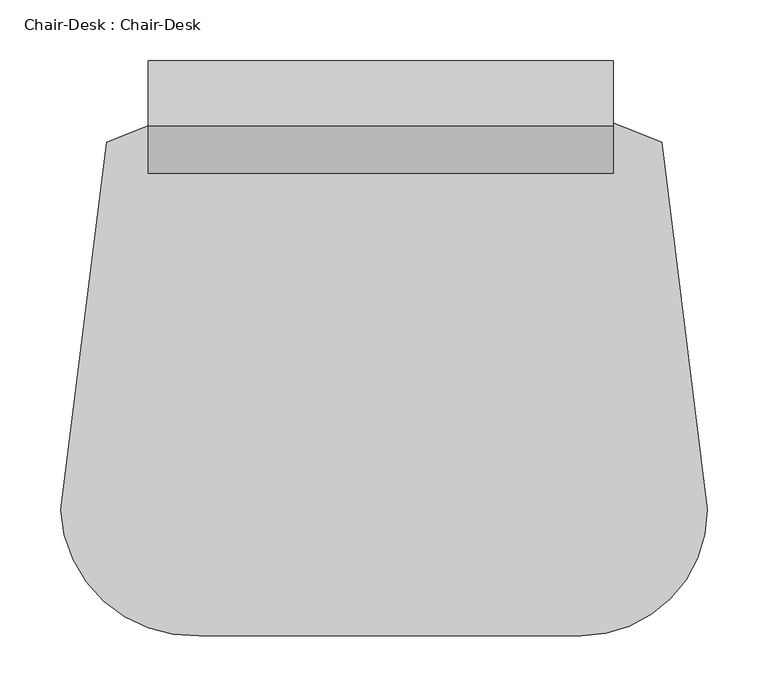
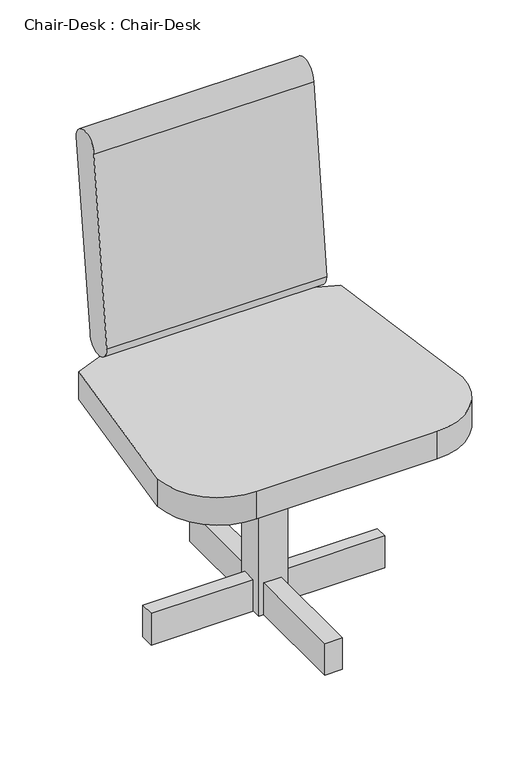
"""IFC4 building model written with IfcOpenShell, lengths in millimetres: furniture geometry, Chair-Desk : Chair-Desk."""

from ifc_helpers import new_model, si_unit, point, frame, frame_2d, origin, origin_with_axes, place, context, project, spatial, polyline, circle_curve, trimmed, segment, composite_curve, outline, extrude, source, transform, mapped, element, save


def chair_desk_chair_desk_f6d25cbe(model_context):
    return source(origin(), model_context, "Body", "SweptSolid", [
        extrude(outline(composite_curve([segment(polyline([(-266.4057871, -302.4462968), (-228.6, 0.0)]), True, "CONTINUOUS"), segment(trimmed(circle_curve(frame_2d((0.0, -446.8941036)), 501.9684252), [point((-228.6, 0.0))], [point((228.6, 0.0))], False, "CARTESIAN"), True, "CONTINUOUS"), segment(polyline([(228.6, 0.0), (266.2067116, -302.4462968)]), True, "CONTINUOUS"), segment(trimmed(circle_curve(frame_2d((162.2530084, -302.4462968)), 103.9537032), [point((266.2067116, -302.4462968))], [point((162.2530084, -406.4))], False, "CARTESIAN"), True, "CONTINUOUS"), segment(polyline([(162.2530084, -406.4), (-152.4, -406.4)]), True, "CONTINUOUS"), segment(trimmed(circle_curve(frame_2d((-157.1362322, -297.1024212)), 109.4001491), [point((-152.4, -406.4))], [point((-266.4057871, -302.4462968))], False, "CARTESIAN"), True, "CONTINUOUS")], self_intersect=False)), frame((0.0, 0.0, 355.6), z_axis=(0.0, 0.0, 1.0), x_axis=(1.0, 0.0, 0.0)), (0.0, 0.0, 1.0), 50.8),
        extrude(outline(composite_curve([segment(trimmed(circle_curve(frame_2d((40.4206181, 787.4)), 26.7884929), [point((13.6321252, 787.4))], [point((67.209111, 787.4))], False, "CARTESIAN"), True, "CONTINUOUS"), segment(polyline([(67.209111, 787.4), (25.4, 451.3880753)]), True, "CONTINUOUS"), segment(trimmed(circle_curve(frame_2d((-0.0761963, 451.3880753)), 25.4761963), [point((25.4, 451.3880753))], [point((-25.5523927, 451.3880753))], False, "CARTESIAN"), True, "CONTINUOUS"), segment(polyline([(-25.5523927, 451.3880753), (13.6321252, 787.4)]), True, "CONTINUOUS")], self_intersect=False)), frame((-194.3643056, 0.0, 0.0), z_axis=(1.0, 0.0, 0.0), x_axis=(0.0, 1.0, 0.0)), (0.0, 0.0, 1.0), 383.2768056),
        extrude(outline(polyline([(26.3236364, -190.2690909), (-24.4763636, -190.2690909), (-24.4763636, -139.4690909), (26.3236364, -139.4690909), (26.3236364, -190.2690909)])), origin_with_axes(), (0.0, 0.0, 1.0), 355.6),
        extrude(outline(polyline([(-203.6618182, -175.0290909), (-203.6618182, -150.0462968), (-25.8618182, -150.0462968), (-25.8618182, -175.0290909), (-203.6618182, -175.0290909)])), origin_with_axes(), (0.0, 0.0, 1.0), 58.5040426),
        extrude(outline(polyline([(204.1236364, -175.0290909), (26.7854545, -175.0290909), (26.7854545, -152.4), (204.1236364, -152.4), (204.1236364, -175.0290909)])), origin_with_axes(), (0.0, 0.0, 1.0), 58.5040426),
        extrude(outline(polyline([(-16.1636364, -188.8836364), (14.3163636, -188.8836364), (14.3163636, -374.9517514), (-16.1636364, -374.9517514), (-16.1636364, -188.8836364)])), origin_with_axes(), (0.0, 0.0, 1.0), 58.5040426),
        extrude(outline(polyline([(14.3163636, -136.2363636), (-16.1636364, -136.2363636), (-16.1636364, 33.2509091), (14.3163636, 33.2509091), (14.3163636, -136.2363636)])), origin_with_axes(), (0.0, 0.0, 1.0), 58.5040426),
    ])


if __name__ == "__main__":
    model = new_model("IFC4")
    model_context = context("Model", 3, world=origin())
    ifc_project = project(units=[si_unit("LENGTHUNIT", "METRE", prefix="MILLI")], contexts=[model_context])
    site = spatial("IfcSite", under=ifc_project)
    building = spatial("IfcBuilding", under=site)
    placement = place(None, origin())
    chair_desk_chair_desk_shape = chair_desk_chair_desk_f6d25cbe(model_context)
    element("IfcFurniture", 1, ObjectType="Chair-Desk : Chair-Desk", at=placement, inside=building, context=model_context, shape_type="MappedRepresentation", body=[
        mapped(chair_desk_chair_desk_shape, transform((0.0, 0.0, 0.0), x_axis=(1.0, 0.0, 0.0), y_axis=(0.0, 1.0, 0.0), z_axis=(0.0, 0.0, 1.0))),
    ])
    save(model, "model.ifc")

# Revit data of these elements
# Type "Chair-Desk : Chair-Desk"
#   Assembly Code = "E2020200"
#   Seat/Back Material = Textile - Slate Blue
#   Base Material = Steel, Chrome Plated
#   Default Elevation = 0
# Element 1 (IfcFurniture, "Chair-Desk : Chair-Desk")
#   Materials on its faces: "Steel, Chrome Plated", "Textile - Slate Blue"
# Materials
#   "Textile - Slate Blue": class "Fabric", colour RGB 98 102 118, transparency 0
#   "Steel, Chrome Plated": class "Metal", colour RGB 17 17 17, transparency 0, Description = "Chromiuim plated steel", Cost = 0
